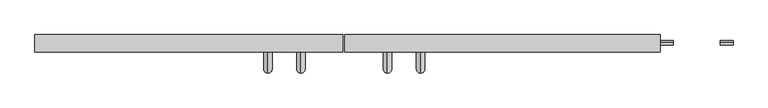
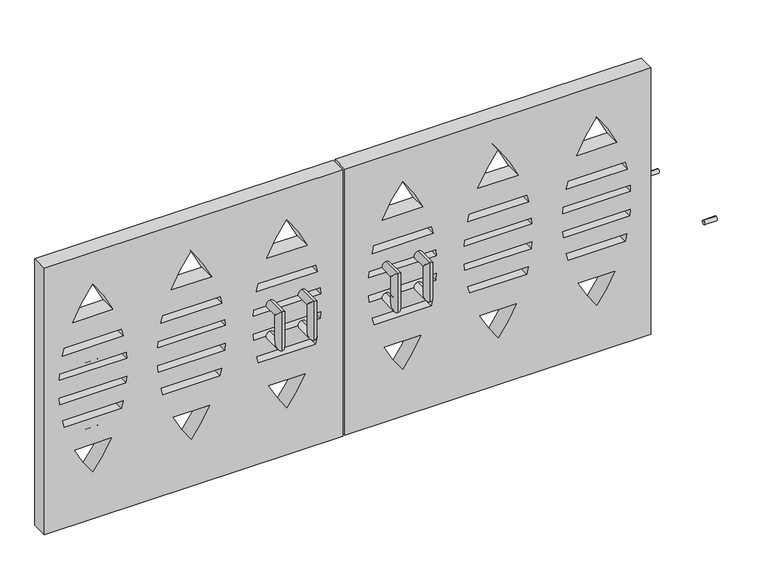
"""IFC4 building model written with IfcOpenShell, lengths in millimetres: proxy geometry."""

from ifc_helpers import new_model, si_unit, point, frame, frame_2d, origin, place, context, project, spatial, polyline, circle_curve, ellipse_curve, trimmed, segment, composite_curve, outline, extrude, source, transform, mapped, element, save
from ifc_brep_helpers import plane_surface, cylinder_surface, advanced_brep


def generic_models_42d6764e(model_context):
    return source(origin(), model_context, "Body", "SolidModel", [
        extrude(outline(polyline([(0.0, -61.4345384), (1727.2, -61.4345384), (1727.2, -1890.2345384), (0.0, -1890.2345384), (0.0, -61.4345384)]), holes=[composite_curve([segment(trimmed(circle_curve(frame_2d((913.3858921, 379.6120442)), 991.7835907), [point((1315.7032602, -526.9062546))], [point((1522.0610264, -403.4264425))], True, "CARTESIAN"), True, "CONTINUOUS"), segment(trimmed(circle_curve(frame_2d((913.3858921, -1186.4649293)), 991.7835907), [point((1522.0610264, -403.4264425))], [point((1315.7032602, -279.9466305))], True, "CARTESIAN"), True, "CONTINUOUS"), segment(polyline([(1315.7032602, -279.9466305), (1315.7032602, -526.9062546)]), True, "CONTINUOUS")], self_intersect=False), composite_curve([segment(trimmed(circle_curve(frame_2d((913.3858921, -1186.4649293)), 991.7835907), [point((1167.7706197, -227.8601613))], [point((1120.5108318, -216.5505258))], True, "CARTESIAN"), True, "CONTINUOUS"), segment(polyline([(1120.5108318, -216.5505258), (1120.5108318, -590.3023593)]), True, "CONTINUOUS"), segment(trimmed(circle_curve(frame_2d((913.3858921, 379.6120442)), 991.7835907), [point((1120.5108318, -590.3023593))], [point((1167.7706197, -578.9927238))], True, "CARTESIAN"), True, "CONTINUOUS"), segment(polyline([(1167.7706197, -578.9927238), (1167.7706197, -227.8601613)]), True, "CONTINUOUS")], self_intersect=False), composite_curve([segment(trimmed(circle_curve(frame_2d((913.3858921, -1186.4649293)), 991.7835907), [point((1008.9376367, -199.2949566))], [point((969.7809206, -196.2860103))], True, "CARTESIAN"), True, "CONTINUOUS"), segment(polyline([(969.7809206, -196.2860103), (969.7809206, -610.5668748)]), True, "CONTINUOUS"), segment(trimmed(circle_curve(frame_2d((913.3858921, 379.6120442)), 991.7835907), [point((969.7809206, -610.5668748))], [point((1008.9376367, -607.5579284))], True, "CARTESIAN"), True, "CONTINUOUS"), segment(polyline([(1008.9376367, -607.5579284), (1008.9376367, -199.2949566)]), True, "CONTINUOUS")], self_intersect=False), composite_curve([segment(trimmed(circle_curve(frame_2d((913.3858921, -1186.4649293)), 991.7835907), [point((853.4628105, -196.4932554))], [point((811.4921317, -199.9293991))], True, "CARTESIAN"), True, "CONTINUOUS"), segment(polyline([(811.4921317, -199.9293991), (811.4921317, -606.923486)]), True, "CONTINUOUS"), segment(trimmed(circle_curve(frame_2d((913.3858921, 379.6120442)), 991.7835907), [point((811.4921317, -606.923486))], [point((853.4628105, -610.3596297))], True, "CARTESIAN"), True, "CONTINUOUS"), segment(polyline([(853.4628105, -610.3596297), (853.4628105, -196.4932554)]), True, "CONTINUOUS")], self_intersect=False), composite_curve([segment(trimmed(circle_curve(frame_2d((913.3858921, -1186.4649293)), 991.7835907), [point((700.6764218, -217.7599319))], [point((655.683383, -228.7467517))], True, "CARTESIAN"), True, "CONTINUOUS"), segment(polyline([(655.683383, -228.7467517), (655.683383, -578.1061333)]), True, "CONTINUOUS"), segment(trimmed(circle_curve(frame_2d((913.3858921, 379.6120442)), 991.7835907), [point((655.683383, -578.1061333))], [point((700.6764218, -589.0929532))], True, "CARTESIAN"), True, "CONTINUOUS"), segment(polyline([(700.6764218, -589.0929532), (700.6764218, -217.7599319)]), True, "CONTINUOUS")], self_intersect=False), composite_curve([segment(trimmed(circle_curve(frame_2d((913.3858921, -1186.4649293)), 991.7835907), [point((485.5755246, -291.6951375))], [point((304.7107578, -403.4264425))], True, "CARTESIAN"), True, "CONTINUOUS"), segment(trimmed(circle_curve(frame_2d((913.3858921, 379.6120442)), 991.7835907), [point((304.7107578, -403.4264425))], [point((485.5755246, -515.1577476))], True, "CARTESIAN"), True, "CONTINUOUS"), segment(polyline([(485.5755246, -515.1577476), (485.5755246, -291.6951375)]), True, "CONTINUOUS")], self_intersect=False), composite_curve([segment(polyline([(1315.7032602, -865.6774949), (1315.7032602, -1112.6371191)]), True, "CONTINUOUS"), segment(trimmed(circle_curve(frame_2d((913.3858921, -206.1188202)), 991.7835907), [point((1315.7032602, -1112.6371191))], [point((1522.0610264, -989.157307))], True, "CARTESIAN"), True, "CONTINUOUS"), segment(trimmed(circle_curve(frame_2d((913.3858921, -1772.1957937)), 991.7835907), [point((1522.0610264, -989.157307))], [point((1315.7032602, -865.6774949))], True, "CARTESIAN"), True, "CONTINUOUS")], self_intersect=False), composite_curve([segment(polyline([(1167.7706197, -1164.7235882), (1167.7706197, -813.5910257)]), True, "CONTINUOUS"), segment(trimmed(circle_curve(frame_2d((913.3858921, -1772.1957937)), 991.7835907), [point((1167.7706197, -813.5910257))], [point((1120.5108318, -802.2813902))], True, "CARTESIAN"), True, "CONTINUOUS"), segment(polyline([(1120.5108318, -802.2813902), (1120.5108318, -1176.0332237)]), True, "CONTINUOUS"), segment(trimmed(circle_curve(frame_2d((913.3858921, -206.1188202)), 991.7835907), [point((1120.5108318, -1176.0332237))], [point((1167.7706197, -1164.7235882))], True, "CARTESIAN"), True, "CONTINUOUS")], self_intersect=False), composite_curve([segment(polyline([(1008.9376367, -1193.2887929), (1008.9376367, -785.0258211)]), True, "CONTINUOUS"), segment(trimmed(circle_curve(frame_2d((913.3858921, -1772.1957937)), 991.7835907), [point((1008.9376367, -785.0258211))], [point((969.7809206, -782.0168748))], True, "CARTESIAN"), True, "CONTINUOUS"), segment(polyline([(969.7809206, -782.0168748), (969.7809206, -1196.2977392)]), True, "CONTINUOUS"), segment(trimmed(circle_curve(frame_2d((913.3858921, -206.1188202)), 991.7835907), [point((969.7809206, -1196.2977392))], [point((1008.9376367, -1193.2887929))], True, "CARTESIAN"), True, "CONTINUOUS")], self_intersect=False), composite_curve([segment(polyline([(853.4628105, -1196.0904941), (853.4628105, -782.2241198)]), True, "CONTINUOUS"), segment(trimmed(circle_curve(frame_2d((913.3858921, -1772.1957937)), 991.7835907), [point((853.4628105, -782.2241198))], [point((811.4921317, -785.6602635))], True, "CARTESIAN"), True, "CONTINUOUS"), segment(polyline([(811.4921317, -785.6602635), (811.4921317, -1192.6543504)]), True, "CONTINUOUS"), segment(trimmed(circle_curve(frame_2d((913.3858921, -206.1188202)), 991.7835907), [point((811.4921317, -1192.6543504))], [point((853.4628105, -1196.0904941))], True, "CARTESIAN"), True, "CONTINUOUS")], self_intersect=False), composite_curve([segment(polyline([(700.6764218, -1174.8238176), (700.6764218, -803.4907963)]), True, "CONTINUOUS"), segment(trimmed(circle_curve(frame_2d((913.3858921, -1772.1957937)), 991.7835907), [point((700.6764218, -803.4907963))], [point((655.683383, -814.4776162))], True, "CARTESIAN"), True, "CONTINUOUS"), segment(polyline([(655.683383, -814.4776162), (655.683383, -1163.8369978)]), True, "CONTINUOUS"), segment(trimmed(circle_curve(frame_2d((913.3858921, -206.1188202)), 991.7835907), [point((655.683383, -1163.8369978))], [point((700.6764218, -1174.8238176))], True, "CARTESIAN"), True, "CONTINUOUS")], self_intersect=False), composite_curve([segment(polyline([(485.5755246, -1100.888612), (485.5755246, -877.4260019)]), True, "CONTINUOUS"), segment(trimmed(circle_curve(frame_2d((913.3858921, -1772.1957937)), 991.7835907), [point((485.5755246, -877.4260019))], [point((304.7107578, -989.157307))], True, "CARTESIAN"), True, "CONTINUOUS"), segment(trimmed(circle_curve(frame_2d((913.3858921, -206.1188202)), 991.7835907), [point((304.7107578, -989.157307))], [point((485.5755246, -1100.888612))], True, "CARTESIAN"), True, "CONTINUOUS")], self_intersect=False), composite_curve([segment(trimmed(circle_curve(frame_2d((913.3858921, -810.8996847)), 991.7835907), [point((1315.7032602, -1717.4179835))], [point((1522.0610264, -1593.9381714))], True, "CARTESIAN"), True, "CONTINUOUS"), segment(trimmed(circle_curve(frame_2d((913.3858921, -2376.9766581)), 991.7835907), [point((1522.0610264, -1593.9381714))], [point((1315.7032602, -1470.4583593))], True, "CARTESIAN"), True, "CONTINUOUS"), segment(polyline([(1315.7032602, -1470.4583593), (1315.7032602, -1717.4179835)]), True, "CONTINUOUS")], self_intersect=False), composite_curve([segment(trimmed(circle_curve(frame_2d((913.3858921, -2376.9766581)), 991.7835907), [point((1167.7706197, -1418.3718902))], [point((1120.5108318, -1407.0622546))], True, "CARTESIAN"), True, "CONTINUOUS"), segment(polyline([(1120.5108318, -1407.0622546), (1120.5108318, -1780.8140882)]), True, "CONTINUOUS"), segment(trimmed(circle_curve(frame_2d((913.3858921, -810.8996847)), 991.7835907), [point((1120.5108318, -1780.8140882))], [point((1167.7706197, -1769.5044526))], True, "CARTESIAN"), True, "CONTINUOUS"), segment(polyline([(1167.7706197, -1769.5044526), (1167.7706197, -1418.3718902)]), True, "CONTINUOUS")], self_intersect=False), composite_curve([segment(trimmed(circle_curve(frame_2d((913.3858921, -2376.9766581)), 991.7835907), [point((1008.9376367, -1389.8066855))], [point((969.7809206, -1386.7977392))], True, "CARTESIAN"), True, "CONTINUOUS"), segment(polyline([(969.7809206, -1386.7977392), (969.7809206, -1801.0786036)]), True, "CONTINUOUS"), segment(trimmed(circle_curve(frame_2d((913.3858921, -810.8996847)), 991.7835907), [point((969.7809206, -1801.0786036))], [point((1008.9376367, -1798.0696573))], True, "CARTESIAN"), True, "CONTINUOUS"), segment(polyline([(1008.9376367, -1798.0696573), (1008.9376367, -1389.8066855)]), True, "CONTINUOUS")], self_intersect=False), composite_curve([segment(trimmed(circle_curve(frame_2d((913.3858921, -2376.9766581)), 991.7835907), [point((853.4628105, -1387.0049843))], [point((811.4921317, -1390.4411279))], True, "CARTESIAN"), True, "CONTINUOUS"), segment(polyline([(811.4921317, -1390.4411279), (811.4921317, -1797.4352149)]), True, "CONTINUOUS"), segment(trimmed(circle_curve(frame_2d((913.3858921, -810.8996847)), 991.7835907), [point((811.4921317, -1797.4352149))], [point((853.4628105, -1800.8713585))], True, "CARTESIAN"), True, "CONTINUOUS"), segment(polyline([(853.4628105, -1800.8713585), (853.4628105, -1387.0049843)]), True, "CONTINUOUS")], self_intersect=False), composite_curve([segment(trimmed(circle_curve(frame_2d((913.3858921, -2376.9766581)), 991.7835907), [point((700.6764218, -1408.2716607))], [point((655.683383, -1419.2584806))], True, "CARTESIAN"), True, "CONTINUOUS"), segment(polyline([(655.683383, -1419.2584806), (655.683383, -1768.6178622)]), True, "CONTINUOUS"), segment(trimmed(circle_curve(frame_2d((913.3858921, -810.8996847)), 991.7835907), [point((655.683383, -1768.6178622))], [point((700.6764218, -1779.6046821))], True, "CARTESIAN"), True, "CONTINUOUS"), segment(polyline([(700.6764218, -1779.6046821), (700.6764218, -1408.2716607)]), True, "CONTINUOUS")], self_intersect=False), composite_curve([segment(trimmed(circle_curve(frame_2d((913.3858921, -2376.9766581)), 991.7835907), [point((485.5755246, -1482.2068664))], [point((304.7107578, -1593.9381714))], True, "CARTESIAN"), True, "CONTINUOUS"), segment(trimmed(circle_curve(frame_2d((913.3858921, -810.8996847)), 991.7835907), [point((304.7107578, -1593.9381714))], [point((485.5755246, -1705.6694764))], True, "CARTESIAN"), True, "CONTINUOUS"), segment(polyline([(485.5755246, -1705.6694764), (485.5755246, -1482.2068664)]), True, "CONTINUOUS")], self_intersect=False)]), frame((0.0, -101.6, 0.0), z_axis=(0.0, 1.0, 0.0), x_axis=(0.0, 0.0, 1.0)), (0.0, 0.0, 1.0), 101.6),
        extrude(outline(polyline([(1727.2, 1827.666195), (1727.2, -47.7825897), (0.0, -47.7825897), (0.0, 1827.666195), (1727.2, 1827.666195)]), holes=[composite_curve([segment(polyline([(1315.7032602, 429.4371778), (1315.7032602, 182.4775536)]), True, "CONTINUOUS"), segment(trimmed(circle_curve(frame_2d((913.3858921, 1088.9958525)), 991.7835907), [point((1315.7032602, 182.4775536))], [point((1522.0610264, 305.9573657))], True, "CARTESIAN"), True, "CONTINUOUS"), segment(trimmed(circle_curve(frame_2d((913.3858921, -477.081121)), 991.7835907), [point((1522.0610264, 305.9573657))], [point((1315.7032602, 429.4371778))], True, "CARTESIAN"), True, "CONTINUOUS")], self_intersect=False), composite_curve([segment(polyline([(1167.7706197, 130.3910845), (1167.7706197, 481.5236469)]), True, "CONTINUOUS"), segment(trimmed(circle_curve(frame_2d((913.3858921, -477.081121)), 991.7835907), [point((1167.7706197, 481.5236469))], [point((1120.5108318, 492.8332825))], True, "CARTESIAN"), True, "CONTINUOUS"), segment(polyline([(1120.5108318, 492.8332825), (1120.5108318, 119.081449)]), True, "CONTINUOUS"), segment(trimmed(circle_curve(frame_2d((913.3858921, 1088.9958525)), 991.7835907), [point((1120.5108318, 119.081449))], [point((1167.7706197, 130.3910845))], True, "CARTESIAN"), True, "CONTINUOUS")], self_intersect=False), composite_curve([segment(polyline([(1008.9376367, 101.8258798), (1008.9376367, 510.0888516)]), True, "CONTINUOUS"), segment(trimmed(circle_curve(frame_2d((913.3858921, -477.081121)), 991.7835907), [point((1008.9376367, 510.0888516))], [point((969.7809206, 513.0977979))], True, "CARTESIAN"), True, "CONTINUOUS"), segment(polyline([(969.7809206, 513.0977979), (969.7809206, 98.8169335)]), True, "CONTINUOUS"), segment(trimmed(circle_curve(frame_2d((913.3858921, 1088.9958525)), 991.7835907), [point((969.7809206, 98.8169335))], [point((1008.9376367, 101.8258798))], True, "CARTESIAN"), True, "CONTINUOUS")], self_intersect=False), composite_curve([segment(polyline([(853.4628105, 99.0241786), (853.4628105, 512.8905529)]), True, "CONTINUOUS"), segment(trimmed(circle_curve(frame_2d((913.3858921, -477.081121)), 991.7835907), [point((853.4628105, 512.8905529))], [point((811.4921317, 509.4544092))], True, "CARTESIAN"), True, "CONTINUOUS"), segment(polyline([(811.4921317, 509.4544092), (811.4921317, 102.4603222)]), True, "CONTINUOUS"), segment(trimmed(circle_curve(frame_2d((913.3858921, 1088.9958525)), 991.7835907), [point((811.4921317, 102.4603222))], [point((853.4628105, 99.0241786))], True, "CARTESIAN"), True, "CONTINUOUS")], self_intersect=False), composite_curve([segment(polyline([(700.6764218, 120.290855), (700.6764218, 491.6238764)]), True, "CONTINUOUS"), segment(trimmed(circle_curve(frame_2d((913.3858921, -477.081121)), 991.7835907), [point((700.6764218, 491.6238764))], [point((655.683383, 480.6370565))], True, "CARTESIAN"), True, "CONTINUOUS"), segment(polyline([(655.683383, 480.6370565), (655.683383, 131.2776749)]), True, "CONTINUOUS"), segment(trimmed(circle_curve(frame_2d((913.3858921, 1088.9958525)), 991.7835907), [point((655.683383, 131.2776749))], [point((700.6764218, 120.290855))], True, "CARTESIAN"), True, "CONTINUOUS")], self_intersect=False), composite_curve([segment(polyline([(485.5755246, 194.2260607), (485.5755246, 417.6886707)]), True, "CONTINUOUS"), segment(trimmed(circle_curve(frame_2d((913.3858921, -477.081121)), 991.7835907), [point((485.5755246, 417.6886707))], [point((304.7107578, 305.9573657))], True, "CARTESIAN"), True, "CONTINUOUS"), segment(trimmed(circle_curve(frame_2d((913.3858921, 1088.9958525)), 991.7835907), [point((304.7107578, 305.9573657))], [point((485.5755246, 194.2260607))], True, "CARTESIAN"), True, "CONTINUOUS")], self_intersect=False), composite_curve([segment(trimmed(circle_curve(frame_2d((913.3858921, 1674.7267169)), 991.7835907), [point((1315.7032602, 768.2084181))], [point((1522.0610264, 891.6882301))], True, "CARTESIAN"), True, "CONTINUOUS"), segment(trimmed(circle_curve(frame_2d((913.3858921, 108.6497434)), 991.7835907), [point((1522.0610264, 891.6882301))], [point((1315.7032602, 1015.1680422))], True, "CARTESIAN"), True, "CONTINUOUS"), segment(polyline([(1315.7032602, 1015.1680422), (1315.7032602, 768.2084181)]), True, "CONTINUOUS")], self_intersect=False), composite_curve([segment(trimmed(circle_curve(frame_2d((913.3858921, 108.6497434)), 991.7835907), [point((1167.7706197, 1067.2545114))], [point((1120.5108318, 1078.5641469))], True, "CARTESIAN"), True, "CONTINUOUS"), segment(polyline([(1120.5108318, 1078.5641469), (1120.5108318, 704.8123134)]), True, "CONTINUOUS"), segment(trimmed(circle_curve(frame_2d((913.3858921, 1674.7267169)), 991.7835907), [point((1120.5108318, 704.8123134))], [point((1167.7706197, 716.1219489))], True, "CARTESIAN"), True, "CONTINUOUS"), segment(polyline([(1167.7706197, 716.1219489), (1167.7706197, 1067.2545114)]), True, "CONTINUOUS")], self_intersect=False), composite_curve([segment(trimmed(circle_curve(frame_2d((913.3858921, 108.6497434)), 991.7835907), [point((1008.9376367, 1095.819716))], [point((969.7809206, 1098.8286624))], True, "CARTESIAN"), True, "CONTINUOUS"), segment(polyline([(969.7809206, 1098.8286624), (969.7809206, 684.5477979)]), True, "CONTINUOUS"), segment(trimmed(circle_curve(frame_2d((913.3858921, 1674.7267169)), 991.7835907), [point((969.7809206, 684.5477979))], [point((1008.9376367, 687.5567442))], True, "CARTESIAN"), True, "CONTINUOUS"), segment(polyline([(1008.9376367, 687.5567442), (1008.9376367, 1095.819716)]), True, "CONTINUOUS")], self_intersect=False), composite_curve([segment(trimmed(circle_curve(frame_2d((913.3858921, 108.6497434)), 991.7835907), [point((853.4628105, 1098.6214173))], [point((811.4921317, 1095.1852736))], True, "CARTESIAN"), True, "CONTINUOUS"), segment(polyline([(811.4921317, 1095.1852736), (811.4921317, 688.1911867)]), True, "CONTINUOUS"), segment(trimmed(circle_curve(frame_2d((913.3858921, 1674.7267169)), 991.7835907), [point((811.4921317, 688.1911867))], [point((853.4628105, 684.755043))], True, "CARTESIAN"), True, "CONTINUOUS"), segment(polyline([(853.4628105, 684.755043), (853.4628105, 1098.6214173)]), True, "CONTINUOUS")], self_intersect=False), composite_curve([segment(trimmed(circle_curve(frame_2d((913.3858921, 108.6497434)), 991.7835907), [point((700.6764218, 1077.3547408))], [point((655.683383, 1066.3679209))], True, "CARTESIAN"), True, "CONTINUOUS"), segment(polyline([(655.683383, 1066.3679209), (655.683383, 717.0085394)]), True, "CONTINUOUS"), segment(trimmed(circle_curve(frame_2d((913.3858921, 1674.7267169)), 991.7835907), [point((655.683383, 717.0085394))], [point((700.6764218, 706.0217195))], True, "CARTESIAN"), True, "CONTINUOUS"), segment(polyline([(700.6764218, 706.0217195), (700.6764218, 1077.3547408)]), True, "CONTINUOUS")], self_intersect=False), composite_curve([segment(trimmed(circle_curve(frame_2d((913.3858921, 108.6497434)), 991.7835907), [point((485.5755246, 1003.4195352))], [point((304.7107578, 891.6882301))], True, "CARTESIAN"), True, "CONTINUOUS"), segment(trimmed(circle_curve(frame_2d((913.3858921, 1674.7267169)), 991.7835907), [point((304.7107578, 891.6882301))], [point((485.5755246, 779.9569251))], True, "CARTESIAN"), True, "CONTINUOUS"), segment(polyline([(485.5755246, 779.9569251), (485.5755246, 1003.4195352)]), True, "CONTINUOUS")], self_intersect=False), composite_curve([segment(polyline([(1315.7032602, 1619.9489067), (1315.7032602, 1372.9892825)]), True, "CONTINUOUS"), segment(trimmed(circle_curve(frame_2d((913.3858921, 2279.5075813)), 991.7835907), [point((1315.7032602, 1372.9892825))], [point((1522.0610264, 1496.4690946))], True, "CARTESIAN"), True, "CONTINUOUS"), segment(trimmed(circle_curve(frame_2d((913.3858921, 713.4306078)), 991.7835907), [point((1522.0610264, 1496.4690946))], [point((1315.7032602, 1619.9489067))], True, "CARTESIAN"), True, "CONTINUOUS")], self_intersect=False), composite_curve([segment(polyline([(1167.7706197, 1320.9028134), (1167.7706197, 1672.0353758)]), True, "CONTINUOUS"), segment(trimmed(circle_curve(frame_2d((913.3858921, 713.4306078)), 991.7835907), [point((1167.7706197, 1672.0353758))], [point((1120.5108318, 1683.3450113))], True, "CARTESIAN"), True, "CONTINUOUS"), segment(polyline([(1120.5108318, 1683.3450113), (1120.5108318, 1309.5931778)]), True, "CONTINUOUS"), segment(trimmed(circle_curve(frame_2d((913.3858921, 2279.5075813)), 991.7835907), [point((1120.5108318, 1309.5931778))], [point((1167.7706197, 1320.9028134))], True, "CARTESIAN"), True, "CONTINUOUS")], self_intersect=False), composite_curve([segment(polyline([(1008.9376367, 1292.3376087), (1008.9376367, 1700.6005805)]), True, "CONTINUOUS"), segment(trimmed(circle_curve(frame_2d((913.3858921, 713.4306078)), 991.7835907), [point((1008.9376367, 1700.6005805))], [point((969.7809206, 1703.6095268))], True, "CARTESIAN"), True, "CONTINUOUS"), segment(polyline([(969.7809206, 1703.6095268), (969.7809206, 1289.3286624)]), True, "CONTINUOUS"), segment(trimmed(circle_curve(frame_2d((913.3858921, 2279.5075813)), 991.7835907), [point((969.7809206, 1289.3286624))], [point((1008.9376367, 1292.3376087))], True, "CARTESIAN"), True, "CONTINUOUS")], self_intersect=False), composite_curve([segment(polyline([(853.4628105, 1289.5359074), (853.4628105, 1703.4022817)]), True, "CONTINUOUS"), segment(trimmed(circle_curve(frame_2d((913.3858921, 713.4306078)), 991.7835907), [point((853.4628105, 1703.4022817))], [point((811.4921317, 1699.966138))], True, "CARTESIAN"), True, "CONTINUOUS"), segment(polyline([(811.4921317, 1699.966138), (811.4921317, 1292.9720511)]), True, "CONTINUOUS"), segment(trimmed(circle_curve(frame_2d((913.3858921, 2279.5075813)), 991.7835907), [point((811.4921317, 1292.9720511))], [point((853.4628105, 1289.5359074))], True, "CARTESIAN"), True, "CONTINUOUS")], self_intersect=False), composite_curve([segment(polyline([(700.6764218, 1310.8025839), (700.6764218, 1682.1356052)]), True, "CONTINUOUS"), segment(trimmed(circle_curve(frame_2d((913.3858921, 713.4306078)), 991.7835907), [point((700.6764218, 1682.1356052))], [point((655.683383, 1671.1487854))], True, "CARTESIAN"), True, "CONTINUOUS"), segment(polyline([(655.683383, 1671.1487854), (655.683383, 1321.7894038)]), True, "CONTINUOUS"), segment(trimmed(circle_curve(frame_2d((913.3858921, 2279.5075813)), 991.7835907), [point((655.683383, 1321.7894038))], [point((700.6764218, 1310.8025839))], True, "CARTESIAN"), True, "CONTINUOUS")], self_intersect=False), composite_curve([segment(polyline([(485.5755246, 1384.7377895), (485.5755246, 1608.2003996)]), True, "CONTINUOUS"), segment(trimmed(circle_curve(frame_2d((913.3858921, 713.4306078)), 991.7835907), [point((485.5755246, 1608.2003996))], [point((304.7107578, 1496.4690946))], True, "CARTESIAN"), True, "CONTINUOUS"), segment(trimmed(circle_curve(frame_2d((913.3858921, 2279.5075813)), 991.7835907), [point((304.7107578, 1496.4690946))], [point((485.5755246, 1384.7377895))], True, "CARTESIAN"), True, "CONTINUOUS")], self_intersect=False)]), frame((0.0, -101.6, 0.0), z_axis=(0.0, 1.0, 0.0), x_axis=(0.0, 0.0, 1.0)), (0.0, 0.0, 1.0), 101.6),
        advanced_brep(
        [(205.2654616, -101.6, 1039.4610264), (205.2654616, -101.6, 988.6610264), (205.2654616, -101.6, 785.4610264), (205.2654616, -101.6, 836.2610264), (205.2654616, -228.6, 1039.4610264), (205.2654616, -177.8, 988.6610264), (205.2654616, -228.6, 785.4610264), (205.2654616, -177.8, 836.2610264)],
        [
            (0, 1, circle_curve(frame((205.2654616, -101.6, 1014.0610264), z_axis=(0.0, 1.0, 0.0), x_axis=(0.0, 0.0, -1.0)), 25.4)),
            (1, 0, circle_curve(frame((205.2654616, -101.6, 1014.0610264), z_axis=(0.0, 1.0, 0.0), x_axis=(0.0, 0.0, -1.0)), 25.4)),
            (2, 3, circle_curve(frame((205.2654616, -101.6, 810.8610264), z_axis=(0.0, 1.0, 0.0), x_axis=(0.0, 0.0, 1.0)), 25.4)),
            (3, 2, circle_curve(frame((205.2654616, -101.6, 810.8610264), z_axis=(0.0, 1.0, 0.0), x_axis=(0.0, 0.0, 1.0)), 25.4)),
            (0, 4),
            (4, 5, ellipse_curve(frame((205.2654616, -203.2, 1014.0610264), z_axis=(0.0, 0.7071067811865495, 0.7071067811865455), x_axis=(0.0, 0.7071067811865457, -0.7071067811865493)), 35.9210245, 25.4)),
            (5, 1),
            (5, 4, ellipse_curve(frame((205.2654616, -203.2, 1014.0610264), z_axis=(0.0, 0.7071067811865495, 0.7071067811865455), x_axis=(0.0, 0.7071067811865457, -0.7071067811865493)), 35.9210245, 25.4)),
            (4, 6),
            (6, 7, ellipse_curve(frame((205.2654616, -203.2, 810.8610264), z_axis=(0.0, -0.7071067811865457, 0.7071067811865495), x_axis=(0.0, 0.7071067811865496, 0.7071067811865455)), 35.9210245, 25.4)),
            (7, 5),
            (7, 6, ellipse_curve(frame((205.2654616, -203.2, 810.8610264), z_axis=(0.0, -0.7071067811865457, 0.7071067811865495), x_axis=(0.0, 0.7071067811865496, 0.7071067811865455)), 35.9210245, 25.4)),
            (6, 2),
            (3, 7),
        ],
        [
            plane_surface(frame((205.2654616, -101.6, 1014.0610264), z_axis=(0.0, 1.0, 0.0), x_axis=(1.0, 0.0, 0.0))),
            plane_surface(frame((205.2654616, -101.6, 810.8610264), z_axis=(0.0, 1.0, 0.0), x_axis=(1.0, 0.0, 0.0))),
            cylinder_surface(frame((205.2654616, -101.6, 1014.0610264), z_axis=(0.0, 1.0, 0.0), x_axis=(0.0, 0.0, -1.0)), 25.4),
            cylinder_surface(frame((205.2654616, -203.2, 1014.0610264), z_axis=(0.0, 0.0, 1.0), x_axis=(0.0, 1.0, 0.0)), 25.4),
            cylinder_surface(frame((205.2654616, -203.2, 810.8610264), z_axis=(0.0, -1.0, 0.0), x_axis=(0.0, 0.0, 1.0)), 25.4),
        ],
        [
            (0, [[1, 2]]),
            (1, [[3, 4]]),
            (2, [[-1, 5, 6, 7]]),
            (2, [[-2, -7, 8, -5]]),
            (3, [[-6, 9, 10, 11]]),
            (3, [[-8, -11, 12, -9]]),
            (4, [[-10, 13, -4, 14]]),
            (4, [[-12, -14, -3, -13]]),
        ],
    ),
        advanced_brep(
        [(402.1154616, -101.6, 1039.4610264), (402.1154616, -101.6, 988.6610264), (402.1154616, -101.6, 785.4610264), (402.1154616, -101.6, 836.2610264), (402.1154616, -228.6, 1039.4610264), (402.1154616, -177.8, 988.6610264), (402.1154616, -228.6, 785.4610264), (402.1154616, -177.8, 836.2610264)],
        [
            (0, 1, circle_curve(frame((402.1154616, -101.6, 1014.0610264), z_axis=(0.0, 1.0, 0.0), x_axis=(0.0, 0.0, -1.0)), 25.4)),
            (1, 0, circle_curve(frame((402.1154616, -101.6, 1014.0610264), z_axis=(0.0, 1.0, 0.0), x_axis=(0.0, 0.0, -1.0)), 25.4)),
            (2, 3, circle_curve(frame((402.1154616, -101.6, 810.8610264), z_axis=(0.0, 1.0, 0.0), x_axis=(0.0, 0.0, 1.0)), 25.4)),
            (3, 2, circle_curve(frame((402.1154616, -101.6, 810.8610264), z_axis=(0.0, 1.0, 0.0), x_axis=(0.0, 0.0, 1.0)), 25.4)),
            (0, 4),
            (4, 5, ellipse_curve(frame((402.1154616, -203.2, 1014.0610264), z_axis=(0.0, 0.7071067811865495, 0.7071067811865455), x_axis=(0.0, 0.7071067811865457, -0.7071067811865493)), 35.9210245, 25.4)),
            (5, 1),
            (5, 4, ellipse_curve(frame((402.1154616, -203.2, 1014.0610264), z_axis=(0.0, 0.7071067811865495, 0.7071067811865455), x_axis=(0.0, 0.7071067811865457, -0.7071067811865493)), 35.9210245, 25.4)),
            (4, 6),
            (6, 7, ellipse_curve(frame((402.1154616, -203.2, 810.8610264), z_axis=(0.0, -0.7071067811865457, 0.7071067811865495), x_axis=(0.0, 0.7071067811865496, 0.7071067811865455)), 35.9210245, 25.4)),
            (7, 5),
            (7, 6, ellipse_curve(frame((402.1154616, -203.2, 810.8610264), z_axis=(0.0, -0.7071067811865457, 0.7071067811865495), x_axis=(0.0, 0.7071067811865496, 0.7071067811865455)), 35.9210245, 25.4)),
            (6, 2),
            (3, 7),
        ],
        [
            plane_surface(frame((402.1154616, -101.6, 1014.0610264), z_axis=(0.0, 1.0, 0.0), x_axis=(1.0, 0.0, 0.0))),
            plane_surface(frame((402.1154616, -101.6, 810.8610264), z_axis=(0.0, 1.0, 0.0), x_axis=(1.0, 0.0, 0.0))),
            cylinder_surface(frame((402.1154616, -101.6, 1014.0610264), z_axis=(0.0, 1.0, 0.0), x_axis=(0.0, 0.0, -1.0)), 25.4),
            cylinder_surface(frame((402.1154616, -203.2, 1014.0610264), z_axis=(0.0, 0.0, 1.0), x_axis=(0.0, 1.0, 0.0)), 25.4),
            cylinder_surface(frame((402.1154616, -203.2, 810.8610264), z_axis=(0.0, -1.0, 0.0), x_axis=(0.0, 0.0, 1.0)), 25.4),
        ],
        [
            (0, [[1, 2]]),
            (1, [[3, 4]]),
            (2, [[-1, 5, 6, 7]]),
            (2, [[-2, -7, 8, -5]]),
            (3, [[-6, 9, 10, 11]]),
            (3, [[-8, -11, 12, -9]]),
            (4, [[-10, 13, -4, 14]]),
            (4, [[-12, -14, -3, -13]]),
        ],
    ),
        extrude(outline(composite_curve([segment(trimmed(circle_curve(frame_2d((-47.1865605, 998.9501685)), 12.7), [point((-47.1865605, 1011.6501685))], [point((-47.1865605, 986.2501685))], False, "CARTESIAN"), True, "CONTINUOUS"), segment(trimmed(circle_curve(frame_2d((-47.1865605, 998.9501685)), 12.7), [point((-47.1865605, 986.2501685))], [point((-47.1865605, 1011.6501685))], False, "CARTESIAN"), True, "CONTINUOUS")], self_intersect=False)), frame((1827.666195, 0.0, 0.0), z_axis=(1.0, 0.0, 0.0), x_axis=(0.0, 1.0, 0.0)), (0.0, 0.0, 1.0), 76.2),
        extrude(outline(composite_curve([segment(trimmed(circle_curve(frame_2d((-47.1865605, 567.1501685)), 12.7), [point((-47.1865605, 579.8501685))], [point((-47.1865605, 554.4501685))], False, "CARTESIAN"), True, "CONTINUOUS"), segment(trimmed(circle_curve(frame_2d((-47.1865605, 567.1501685)), 12.7), [point((-47.1865605, 554.4501685))], [point((-47.1865605, 579.8501685))], False, "CARTESIAN"), True, "CONTINUOUS")], self_intersect=False)), frame((2183.266195, 0.0, 0.0), z_axis=(1.0, 0.0, 0.0), x_axis=(0.0, 1.0, 0.0)), (0.0, 0.0, 1.0), 76.2),
        extrude(outline(composite_curve([segment(trimmed(circle_curve(frame_2d((-47.1865605, 998.9501685)), 12.7), [point((-47.1865605, 1011.6501685))], [point((-47.1865605, 986.2501685))], False, "CARTESIAN"), True, "CONTINUOUS"), segment(trimmed(circle_curve(frame_2d((-47.1865605, 998.9501685)), 12.7), [point((-47.1865605, 986.2501685))], [point((-47.1865605, 1011.6501685))], False, "CARTESIAN"), True, "CONTINUOUS")], self_intersect=False)), frame((-1610.8345384, 0.0, 0.0), z_axis=(1.0, 0.0, 0.0), x_axis=(0.0, 1.0, 0.0)), (0.0, 0.0, 1.0), 76.2),
        extrude(outline(composite_curve([segment(trimmed(circle_curve(frame_2d((-47.1865605, 567.1501685)), 12.7), [point((-47.1865605, 579.8501685))], [point((-47.1865605, 554.4501685))], False, "CARTESIAN"), True, "CONTINUOUS"), segment(trimmed(circle_curve(frame_2d((-47.1865605, 567.1501685)), 12.7), [point((-47.1865605, 554.4501685))], [point((-47.1865605, 579.8501685))], False, "CARTESIAN"), True, "CONTINUOUS")], self_intersect=False)), frame((-1610.8345384, 0.0, 0.0), z_axis=(1.0, 0.0, 0.0), x_axis=(0.0, 1.0, 0.0)), (0.0, 0.0, 1.0), 76.2),
        advanced_brep(
        [(-505.9345384, -101.6, 1039.4610264), (-505.9345384, -101.6, 988.6610264), (-505.9345384, -101.6, 785.4610264), (-505.9345384, -101.6, 836.2610264), (-505.9345384, -228.6, 1039.4610264), (-505.9345384, -177.8, 988.6610264), (-505.9345384, -228.6, 785.4610264), (-505.9345384, -177.8, 836.2610264)],
        [
            (0, 1, circle_curve(frame((-505.9345384, -101.6, 1014.0610264), z_axis=(0.0, 1.0, 0.0), x_axis=(0.0, 0.0, -1.0)), 25.4)),
            (1, 0, circle_curve(frame((-505.9345384, -101.6, 1014.0610264), z_axis=(0.0, 1.0, 0.0), x_axis=(0.0, 0.0, -1.0)), 25.4)),
            (2, 3, circle_curve(frame((-505.9345384, -101.6, 810.8610264), z_axis=(0.0, 1.0, 0.0), x_axis=(0.0, 0.0, 1.0)), 25.4)),
            (3, 2, circle_curve(frame((-505.9345384, -101.6, 810.8610264), z_axis=(0.0, 1.0, 0.0), x_axis=(0.0, 0.0, 1.0)), 25.4)),
            (0, 4),
            (4, 5, ellipse_curve(frame((-505.9345384, -203.2, 1014.0610264), z_axis=(0.0, 0.7071067811865495, 0.7071067811865455), x_axis=(0.0, 0.7071067811865457, -0.7071067811865493)), 35.9210245, 25.4)),
            (5, 1),
            (5, 4, ellipse_curve(frame((-505.9345384, -203.2, 1014.0610264), z_axis=(0.0, 0.7071067811865495, 0.7071067811865455), x_axis=(0.0, 0.7071067811865457, -0.7071067811865493)), 35.9210245, 25.4)),
            (4, 6),
            (6, 7, ellipse_curve(frame((-505.9345384, -203.2, 810.8610264), z_axis=(0.0, -0.7071067811865457, 0.7071067811865495), x_axis=(0.0, 0.7071067811865496, 0.7071067811865455)), 35.9210245, 25.4)),
            (7, 5),
            (7, 6, ellipse_curve(frame((-505.9345384, -203.2, 810.8610264), z_axis=(0.0, -0.7071067811865457, 0.7071067811865495), x_axis=(0.0, 0.7071067811865496, 0.7071067811865455)), 35.9210245, 25.4)),
            (6, 2),
            (3, 7),
        ],
        [
            plane_surface(frame((-505.9345384, -101.6, 1014.0610264), z_axis=(0.0, 1.0, 0.0), x_axis=(1.0, 0.0, 0.0))),
            plane_surface(frame((-505.9345384, -101.6, 810.8610264), z_axis=(0.0, 1.0, 0.0), x_axis=(1.0, 0.0, 0.0))),
            cylinder_surface(frame((-505.9345384, -101.6, 1014.0610264), z_axis=(0.0, 1.0, 0.0), x_axis=(0.0, 0.0, -1.0)), 25.4),
            cylinder_surface(frame((-505.9345384, -203.2, 1014.0610264), z_axis=(0.0, 0.0, 1.0), x_axis=(0.0, 1.0, 0.0)), 25.4),
            cylinder_surface(frame((-505.9345384, -203.2, 810.8610264), z_axis=(0.0, -1.0, 0.0), x_axis=(0.0, 0.0, 1.0)), 25.4),
        ],
        [
            (0, [[1, 2]]),
            (1, [[3, 4]]),
            (2, [[-1, 5, 6, 7]]),
            (2, [[-2, -7, 8, -5]]),
            (3, [[-6, 9, 10, 11]]),
            (3, [[-8, -11, 12, -9]]),
            (4, [[-10, 13, -4, 14]]),
            (4, [[-12, -14, -3, -13]]),
        ],
    ),
        advanced_brep(
        [(-309.0845384, -101.6, 1039.4610264), (-309.0845384, -101.6, 988.6610264), (-309.0845384, -101.6, 785.4610264), (-309.0845384, -101.6, 836.2610264), (-309.0845384, -228.6, 1039.4610264), (-309.0845384, -177.8, 988.6610264), (-309.0845384, -228.6, 785.4610264), (-309.0845384, -177.8, 836.2610264)],
        [
            (0, 1, circle_curve(frame((-309.0845384, -101.6, 1014.0610264), z_axis=(0.0, 1.0, 0.0), x_axis=(0.0, 0.0, -1.0)), 25.4)),
            (1, 0, circle_curve(frame((-309.0845384, -101.6, 1014.0610264), z_axis=(0.0, 1.0, 0.0), x_axis=(0.0, 0.0, -1.0)), 25.4)),
            (2, 3, circle_curve(frame((-309.0845384, -101.6, 810.8610264), z_axis=(0.0, 1.0, 0.0), x_axis=(0.0, 0.0, 1.0)), 25.4)),
            (3, 2, circle_curve(frame((-309.0845384, -101.6, 810.8610264), z_axis=(0.0, 1.0, 0.0), x_axis=(0.0, 0.0, 1.0)), 25.4)),
            (0, 4),
            (4, 5, ellipse_curve(frame((-309.0845384, -203.2, 1014.0610264), z_axis=(0.0, 0.7071067811865495, 0.7071067811865455), x_axis=(0.0, 0.7071067811865457, -0.7071067811865493)), 35.9210245, 25.4)),
            (5, 1),
            (5, 4, ellipse_curve(frame((-309.0845384, -203.2, 1014.0610264), z_axis=(0.0, 0.7071067811865495, 0.7071067811865455), x_axis=(0.0, 0.7071067811865457, -0.7071067811865493)), 35.9210245, 25.4)),
            (4, 6),
            (6, 7, ellipse_curve(frame((-309.0845384, -203.2, 810.8610264), z_axis=(0.0, -0.7071067811865457, 0.7071067811865495), x_axis=(0.0, 0.7071067811865496, 0.7071067811865455)), 35.9210245, 25.4)),
            (7, 5),
            (7, 6, ellipse_curve(frame((-309.0845384, -203.2, 810.8610264), z_axis=(0.0, -0.7071067811865457, 0.7071067811865495), x_axis=(0.0, 0.7071067811865496, 0.7071067811865455)), 35.9210245, 25.4)),
            (6, 2),
            (3, 7),
        ],
        [
            plane_surface(frame((-309.0845384, -101.6, 1014.0610264), z_axis=(0.0, 1.0, 0.0), x_axis=(1.0, 0.0, 0.0))),
            plane_surface(frame((-309.0845384, -101.6, 810.8610264), z_axis=(0.0, 1.0, 0.0), x_axis=(1.0, 0.0, 0.0))),
            cylinder_surface(frame((-309.0845384, -101.6, 1014.0610264), z_axis=(0.0, 1.0, 0.0), x_axis=(0.0, 0.0, -1.0)), 25.4),
            cylinder_surface(frame((-309.0845384, -203.2, 1014.0610264), z_axis=(0.0, 0.0, 1.0), x_axis=(0.0, 1.0, 0.0)), 25.4),
            cylinder_surface(frame((-309.0845384, -203.2, 810.8610264), z_axis=(0.0, -1.0, 0.0), x_axis=(0.0, 0.0, 1.0)), 25.4),
        ],
        [
            (0, [[1, 2]]),
            (1, [[3, 4]]),
            (2, [[-1, 5, 6, 7]]),
            (2, [[-2, -7, 8, -5]]),
            (3, [[-6, 9, 10, 11]]),
            (3, [[-8, -11, 12, -9]]),
            (4, [[-10, 13, -4, 14]]),
            (4, [[-12, -14, -3, -13]]),
        ],
    ),
    ])


if __name__ == "__main__":
    model = new_model("IFC4")
    model_context = context("Model", 3, world=origin())
    ifc_project = project(units=[si_unit("LENGTHUNIT", "METRE", prefix="MILLI")], contexts=[model_context])
    site = spatial("IfcSite", under=ifc_project)
    building = spatial("IfcBuilding", under=site)
    placement = place(None, origin())
    generic_models_shape = generic_models_42d6764e(model_context)
    element("IfcBuildingElementProxy", 1, Name="Generic Models", at=placement, inside=building, context=model_context, shape_type="MappedRepresentation", body=[
        mapped(generic_models_shape, transform((0.0, 0.0, 0.0), x_axis=(1.0, 0.0, 0.0), y_axis=(0.0, 1.0, 0.0), z_axis=(0.0, 0.0, 1.0))),
    ])
    save(model, "model.ifc")

# Revit data of these elements
# Type
#   Default Elevation = 0
# Element 1 (IfcBuildingElementProxy)
#   Materials on its faces: "GATE"
# Materials
#   "GATE": class "Generic", colour RGB 120 120 120, transparency 0, Cost = 0
